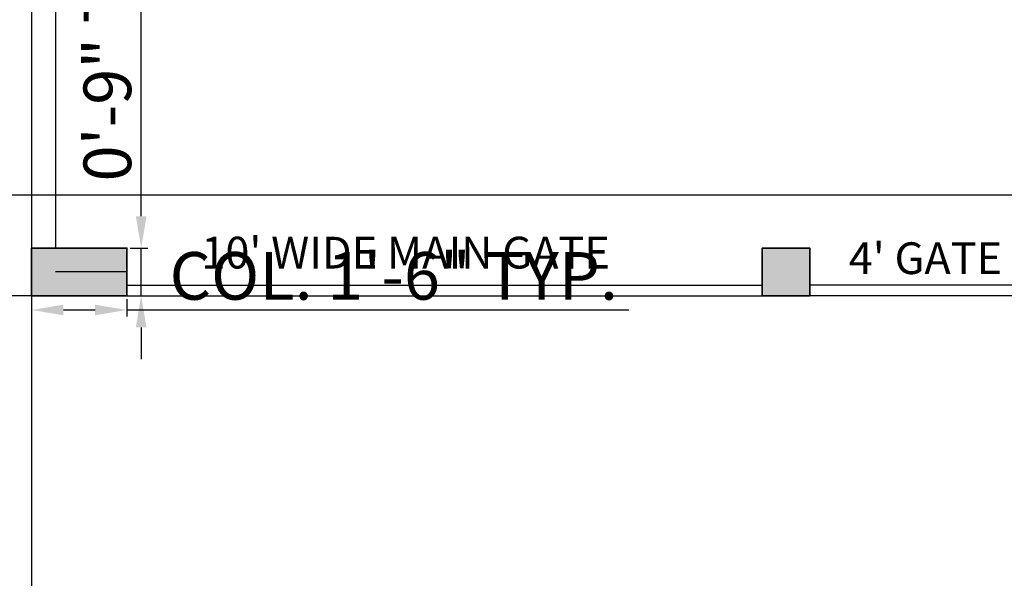
# Model space of a CAD drawing. Units: millimetres. Extents: x 595116 to 630915, y 909473 to 920225.
# Tile 4 of 134: x 629314 to 629500, y 919089 to 919194. Entities that reach past the tile are written whole.
import ezdxf

# ---------------------------------------------------------------- set-up
doc = ezdxf.new("R2010")
doc.units = ezdxf.units.MM
doc.linetypes.add('ACAD_ISO02W100', pattern=[15, 12, -3])
for name, color, linetype, lineweight in [('C-PROP', 7, 'Continuous', 25), ('C-PROP-REF', 240, 'ACAD_ISO02W100', 13), ('Column', 6, 'Continuous', 35), ('Dimension', 3, 'Continuous', 18), ('Text', 7, 'Continuous', 18)]:
    doc.layers.add(name, color=color, linetype=linetype, lineweight=lineweight)
doc.styles.get("Standard").update_dxf_attribs({"font": 'arial.ttf'})
doc.dimstyles.new('ISO-25', dxfattribs={"dimtxt": 9, "dimasz": 6, "dimexe": 1.25, "dimexo": 0.625, "dimtad": 1, "dimlunit": 4, "dimtxsty": 'Standard', "dimcen": 2.5, "dimadec": 0, "dimazin": 0, "dimtfac": 1, "dimtmove": 0, "dimatfit": 3, "dimfxl": 1, "dimarcsym": 0})

# ---------------------------------------------------------------- blocks, each defined once
blk = doc.blocks.new('COLUMN-RECT-18X9')
h = blk.add_hatch(color=256)
h.dxf.hatch_style = 1
h.paths.add_polyline_path([(18, 9), (0, 9), (0, 0), (18, 0)])
blk.add_lwpolyline([(0, 9), (18, 9), (18, 0), (0, 0)], close=True)
blk = doc.blocks.new('*D154')
at = {"layer": 'Defpoints', "color": 0, "transparency": 16777216}
for p in [(629316.04, 919141.93), (629334.04, 919141.93), (629334.04, 919139.23)]:
    blk.add_point(p, dxfattribs=at)
at = {"layer": 'Dimension', "color": 0, "lineweight": -2, "transparency": 16777216}
for p, q in [((629316.04, 919141.3), (629316.04, 919137.98)), ((629334.04, 919141.3), (629334.04, 919137.98)), ((629322.04, 919139.23), (629328.04, 919139.23)), ((629334.04, 919139.23), (629428.88, 919139.23))]:
    blk.add_line(p, q, dxfattribs=at)
at = {"layer": 'Dimension', "color": 0, "transparency": 16777216}
for points in [[(629322.04, 919140.23), (629322.04, 919138.23), (629316.04, 919139.23)], [(629328.04, 919140.23), (629328.04, 919138.23), (629334.04, 919139.23)]]:
    blk.add_solid(points, dxfattribs=at)
at = {"layer": 'Dimension', "color": 0, "transparency": 16777216, "insert": (629384.46, 919144.51), "char_height": 9, "attachment_point": 5}
blk.add_mtext('COL. 1\'-6" TYP.', dxfattribs=at)
blk = doc.blocks.new('*D155')
at = {"layer": 'Defpoints', "color": 0, "transparency": 16777216}
for p in [(629334.04, 919150.93), (629336.74, 919150.93), (629334.04, 919141.93)]:
    blk.add_point(p, dxfattribs=at)
at = {"layer": 'Dimension', "color": 0, "lineweight": -2, "transparency": 16777216}
for p, q in [((629336.74, 919156.93), (629336.74, 919219.04)), ((629334.67, 919150.93), (629337.99, 919150.93)), ((629336.74, 919141.93), (629336.74, 919150.93)), ((629334.67, 919141.93), (629337.99, 919141.93)), ((629336.74, 919135.93), (629336.74, 919129.93))]:
    blk.add_line(p, q, dxfattribs=at)
at = {"layer": 'Dimension', "color": 0, "transparency": 16777216}
for points in [[(629335.74, 919156.93), (629337.74, 919156.93), (629336.74, 919150.93)], [(629335.74, 919135.93), (629337.74, 919135.93), (629336.74, 919141.93)]]:
    blk.add_solid(points, dxfattribs=at)
at = {"layer": 'Dimension', "color": 0, "transparency": 16777216, "insert": (629331.52, 919190.98), "char_height": 9, "attachment_point": 5, "rotation": 90}
blk.add_mtext('0\'-9" TYP.', dxfattribs=at)
blk = doc.blocks.new('*D215')
at = {"layer": 'Defpoints', "color": 0, "transparency": 16777216}
for p in [(629316.04, 919411.83), (629505.04, 919411.83), (629505.04, 918832.38)]:
    blk.add_point(p, dxfattribs=at)
at = {"layer": 'Dimension', "color": 0, "lineweight": -2, "transparency": 16777216}
for p, q in [((629316.04, 919411.2), (629316.04, 918831.13)), ((629505.04, 919411.2), (629505.04, 918831.13)), ((629322.04, 918832.38), (629499.04, 918832.38))]:
    blk.add_line(p, q, dxfattribs=at)
at = {"layer": 'Dimension', "color": 0, "transparency": 16777216}
for points in [[(629322.04, 918833.38), (629322.04, 918831.38), (629316.04, 918832.38)], [(629499.04, 918833.38), (629499.04, 918831.38), (629505.04, 918832.38)]]:
    blk.add_solid(points, dxfattribs=at)
at = {"layer": 'Dimension', "color": 0, "transparency": 16777216, "insert": (629410.54, 918837.6), "char_height": 9, "attachment_point": 5}
blk.add_mtext('15\'-9"', dxfattribs=at)
blk = doc.blocks.new('*D221')
at = {"layer": 'Defpoints', "color": 0, "transparency": 16777216}
for p in [(629511.27, 919302.01), (629155.38, 919160.92), (629511.27, 919160.92)]:
    blk.add_point(p, dxfattribs=at)
at = {"layer": 'Dimension', "color": 0, "lineweight": -2, "transparency": 16777216}
for p, q in [((629510.65, 919302.01), (629154.13, 919302.01)), ((629155.38, 919296.01), (629155.38, 919166.92)), ((629510.65, 919160.92), (629154.13, 919160.92))]:
    blk.add_line(p, q, dxfattribs=at)
at = {"layer": 'Dimension', "color": 0, "transparency": 16777216}
for points in [[(629154.38, 919296.01), (629156.38, 919296.01), (629155.38, 919302.01)], [(629154.38, 919166.92), (629156.38, 919166.92), (629155.38, 919160.92)]]:
    blk.add_solid(points, dxfattribs=at)
at = {"layer": 'Dimension', "color": 0, "transparency": 16777216, "insert": (629150.16, 919231.46), "char_height": 9, "attachment_point": 5, "rotation": 90}
blk.add_mtext('11\'-9"', dxfattribs=at)

msp = doc.modelspace()

# ---------------------------------------------------------------- hatches: boundary and pattern name
at = {"layer": 'Column'}
h = msp.add_hatch(color=256, dxfattribs=at)
h.dxf.hatch_style = 1
h.paths.add_polyline_path([(629463.041, 919150.928), (629454.041, 919150.928), (629454.041, 919141.928), (629463.041, 919141.928)])

# ---------------------------------------------------------------- linework, layer by layer
at = {"layer": 'C-PROP'}
for p, q in [((629320.541, 919345.928), (629320.541, 919150.928)), ((629334.041, 919150.928), (629334.041, 919141.928)), ((629463.041, 919150.928), (629454.041, 919150.928)), ((629334.041, 919146.428), (629320.541, 919146.428)), ((629334.041, 919143.928), (629454.041, 919143.928)), ((629511.041, 919143.928), (629463.041, 919143.928)), ((629334.041, 919141.928), (629454.041, 919141.928)), ((629511.041, 919141.928), (629463.041, 919141.928))]:
    msp.add_line(p, q, dxfattribs=at)
msp.add_lwpolyline([(629334.041, 919141.928), (629311.541, 919141.928)], dxfattribs=at)
at = {"layer": 'C-PROP-REF'}
for p, q in [((629316.041, 919146.428), (629316.041, 920084.928)), ((629334.041, 919141.928), (629316.041, 919141.928))]:
    msp.add_line(p, q, dxfattribs=at)
at = {"layer": 'Column'}
msp.add_lwpolyline([(629454.041, 919150.928), (629454.041, 919141.928), (629463.041, 919141.928), (629454.041, 919141.928), (629454.041, 919150.928), (629463.041, 919150.928), (629463.041, 919141.928)], dxfattribs=at)

# ---------------------------------------------------------------- block references
msp.add_blockref('COLUMN-RECT-18X9', (629316.041, 919141.928), dxfattribs=at)

# ---------------------------------------------------------------- texts
at = {"layer": 'Text', "char_height": 6, "attachment_point": 1}
for s, insert in [("{10' WIDE MAIN GATE}", (629348.097, 919153.067)), ("{ 4' GATE}", (629468.555, 919152.013))]:
    msp.add_mtext_dynamic_manual_height_columns(s, width=83.57324, gutter_width=12.5, heights=[0], dxfattribs=dict(at, insert=insert))

# ---------------------------------------------------------------- dimensions: what is measured, and where the dimension line sits
at = {"layer": 'Dimension'}
dim = msp.add_linear_dim(base=(629505.041, 918832.378), p1=(629316.041, 919411.828), p2=(629505.041, 919411.828), dimstyle='ISO-25', override={"dimdec": 1, "dimlfac": 1, "dimrnd": 0, "dimzin": 1, "dimdsep": 46, "dimlunit": 4, "dimfrac": 2}, dxfattribs=at)
dim.commit()
dim.dimension.update_dxf_attribs({"geometry": '*D215', "text_midpoint": (629410.541, 918837.598)})
dim = msp.add_linear_dim(base=(629155.382, 919160.917), p1=(629511.274, 919302.009), p2=(629511.274, 919160.917), angle=90, dimstyle='ISO-25', override={"dimdec": 1, "dimlfac": 1, "dimrnd": 0, "dimzin": 1, "dimdsep": 46, "dimlunit": 4, "dimfrac": 2}, dxfattribs=at)
dim.commit()
dim.dimension.update_dxf_attribs({"geometry": '*D221', "text_midpoint": (629150.162, 919231.463)})
dim = msp.add_linear_dim(base=(629336.741, 919150.928), p1=(629334.041, 919141.928), p2=(629334.041, 919150.928), angle=90, text='<> TYP.', dimstyle='ISO-25', override={"dimdec": 1, "dimlfac": 1, "dimrnd": 0, "dimzin": 1, "dimdsep": 46, "dimlunit": 4, "dimfrac": 2}, dxfattribs=at)
dim.commit()
dim.dimension.update_dxf_attribs({"geometry": '*D155', "text_midpoint": (629331.521, 919190.982)})
dim = msp.add_linear_dim(base=(629334.041, 919139.228), p1=(629316.041, 919141.928), p2=(629334.041, 919141.928), text='COL. <> TYP.', dimstyle='ISO-25', override={"dimdec": 1, "dimlfac": 1, "dimrnd": 0, "dimzin": 1, "dimdsep": 46, "dimlunit": 4, "dimfrac": 2}, dxfattribs=at)
dim.commit()
dim.dimension.update_dxf_attribs({"geometry": '*D154', "text_midpoint": (629384.463, 919144.509)})

doc.saveas('drawing.dxf')
